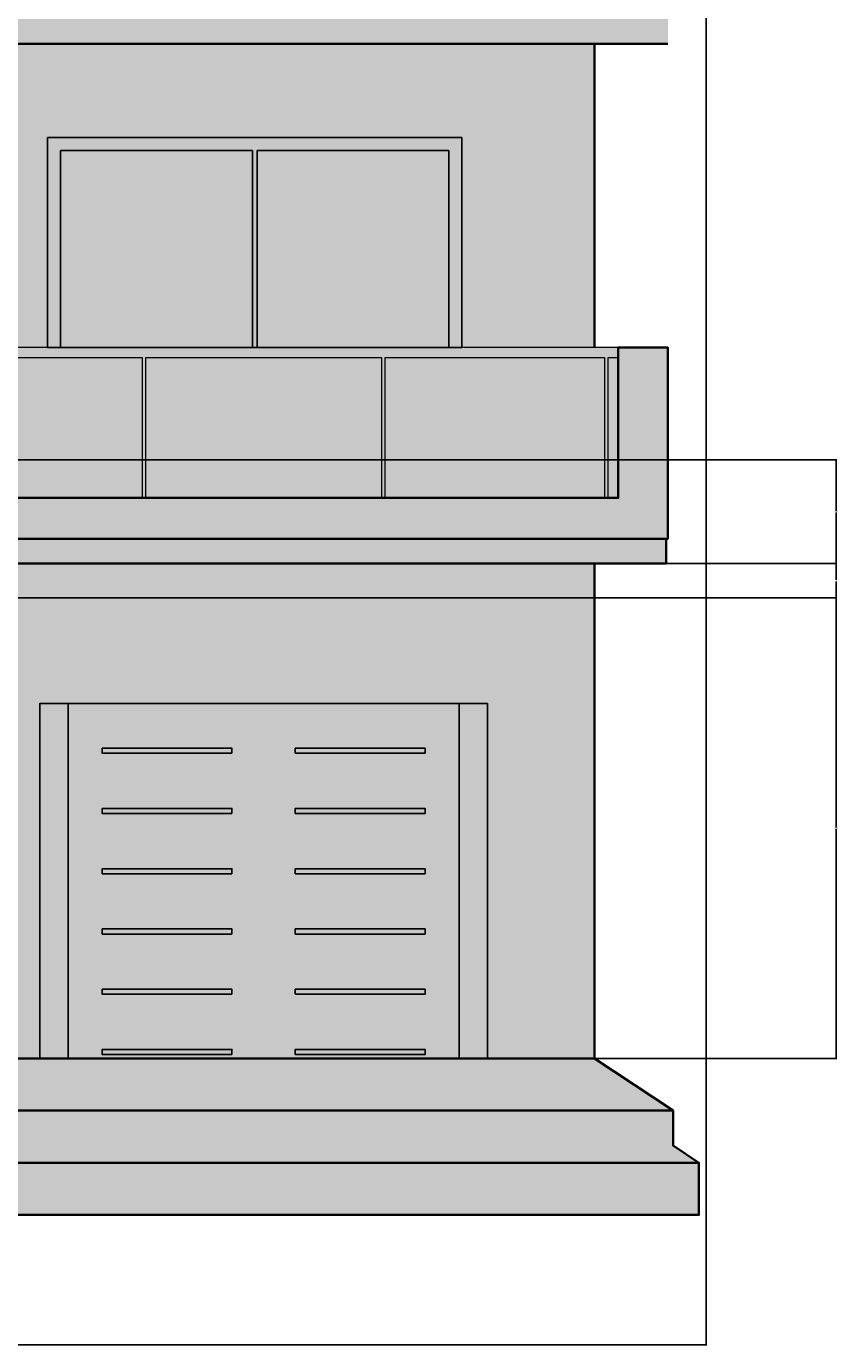
# Model space of a CAD drawing. Units: feet. Extents: x 2893 to 4112, y 897 to 1573.
# Tile 4 of 7: x 3253 to 3449, y 897 to 1217. Entities that reach past the tile are written whole.
import ezdxf

# ---------------------------------------------------------------- set-up
doc = ezdxf.new("R2010")
doc.units = ezdxf.units.FT
for name, color, linetype, lineweight in [('A-ANNO-DIMS', 2, 'Continuous', 18), ('A-DOOR', 3, 'Continuous', 25), ('A-ELEV', 7, 'Continuous', 35), ('A-ELEV-PATT', 8, 'Continuous', 13), ('A-ELEV-RAIL', 4, 'Continuous', 18), ('A-GLAZ', 4, 'Continuous', 25)]:
    doc.layers.add(name, color=color, linetype=linetype, lineweight=lineweight)
doc.styles.get("Standard").update_dxf_attribs({"font": 'arial.ttf'})
doc.dimstyles.get("Standard").update_dxf_attribs({"dimtxt": 0.18, "dimasz": 0.18, "dimexe": 0.18, "dimexo": 0.0625, "dimgap": 0.09, "dimtad": 0, "dimtih": 1, "dimtoh": 1, "dimdec": 1, "dimzin": 0, "dimdsep": 46, "dimlunit": 3, "dimtxsty": 'Standard', "dimcen": 0.09, "dimadec": 0, "dimazin": 0, "dimtfac": 1, "dimtdec": 1, "dimtofl": 0, "dimtmove": 0, "dimatfit": 3, "dimfxl": 1, "dimtolj": 1, "dimtzin": 0, "dimarcsym": 0})

# ---------------------------------------------------------------- blocks, each defined once
blk = doc.blocks.new('WIN-SLIDING')
blk.add_lwpolyline([(100.48, 0), (0, 0), (0, 50.91), (100.48, 50.91)], close=True)
blk.add_lwpolyline([(100.48, 0), (0, 0), (0, 50.91), (100.48, 50.91)], close=True)
blk.add_lwpolyline([(97.33, 0), (97.33, 47.76), (50.81, 47.76), (50.81, 0), (49.67, 0), (49.67, 47.76), (3.15, 47.76), (3.15, 0)])
blk.add_lwpolyline([(97.33, 0), (97.33, 47.76), (50.81, 47.76), (50.81, 0), (49.67, 0), (49.67, 47.76), (3.15, 47.76), (3.15, 0)])
blk = doc.blocks.new('GATE-GARAGE')
for points in [[(108.58, 0), (0, 0), (0, 86.02), (108.58, 86.02)], [(108.58, 0), (0, 0), (0, 86.02), (108.58, 86.02)], [(0, 86.02), (6.87, 86.02), (6.87, 0), (0, 0)], [(0, 86.02), (6.87, 86.02), (6.87, 0), (0, 0)], [(108.58, 86.02), (101.71, 86.02), (101.71, 0), (108.58, 0)], [(108.58, 86.02), (101.71, 86.02), (101.71, 0), (108.58, 0)], [(46.6, 73.98), (15.13, 73.98), (15.13, 75.22), (46.6, 75.22)], [(46.6, 73.98), (15.13, 73.98), (15.13, 75.22), (46.6, 75.22)], [(61.97, 73.98), (93.45, 73.98), (93.45, 75.22), (61.97, 75.22)], [(61.97, 73.98), (93.45, 73.98), (93.45, 75.22), (61.97, 75.22)], [(46.6, 59.37), (15.13, 59.37), (15.13, 60.61), (46.6, 60.61)], [(46.6, 59.37), (15.13, 59.37), (15.13, 60.61), (46.6, 60.61)], [(61.97, 59.37), (93.45, 59.37), (93.45, 60.61), (61.97, 60.61)], [(61.97, 59.37), (93.45, 59.37), (93.45, 60.61), (61.97, 60.61)], [(46.6, 44.76), (15.13, 44.76), (15.13, 46), (46.6, 46)], [(46.6, 44.76), (15.13, 44.76), (15.13, 46), (46.6, 46)], [(61.97, 44.76), (93.45, 44.76), (93.45, 46), (61.97, 46)], [(61.97, 44.76), (93.45, 44.76), (93.45, 46), (61.97, 46)], [(46.6, 30.15), (15.13, 30.15), (15.13, 31.39), (46.6, 31.39)], [(46.6, 30.15), (15.13, 30.15), (15.13, 31.39), (46.6, 31.39)], [(61.97, 30.15), (93.45, 30.15), (93.45, 31.39), (61.97, 31.39)], [(61.97, 30.15), (93.45, 30.15), (93.45, 31.39), (61.97, 31.39)], [(46.6, 15.54), (15.13, 15.54), (15.13, 16.78), (46.6, 16.78)], [(46.6, 15.54), (15.13, 15.54), (15.13, 16.78), (46.6, 16.78)], [(61.97, 15.54), (93.45, 15.54), (93.45, 16.78), (61.97, 16.78)], [(61.97, 15.54), (93.45, 15.54), (93.45, 16.78), (61.97, 16.78)], [(46.6, 0.93), (15.13, 0.93), (15.13, 2.17), (46.6, 2.17)], [(46.6, 0.93), (15.13, 0.93), (15.13, 2.17), (46.6, 2.17)], [(61.97, 0.93), (93.45, 0.93), (93.45, 2.17), (61.97, 2.17)], [(61.97, 0.93), (93.45, 0.93), (93.45, 2.17), (61.97, 2.17)]]:
    blk.add_lwpolyline(points, close=True)
blk = doc.blocks.new('BALCONY-RAIL')
blk.add_lwpolyline([(56.56, 34.07), (3.3, 34.07), (3.3, 0), (2.43, 0), (2.43, 34.07), (0, 34.07), (0, 36.45), (173.25, 36.45), (173.25, 34.07), (170.48, 34.07), (170.48, 0), (169.61, 0), (169.61, 34.07), (115.47, 34.07), (115.47, 0), (114.59, 0), (114.59, 34.07), (57.43, 34.07), (57.43, 0), (56.56, 0)], close=True)
blk.add_lwpolyline([(56.56, 34.07), (3.3, 34.07), (3.3, 0), (2.43, 0), (2.43, 34.07), (0, 34.07), (0, 36.45), (173.25, 36.45), (173.25, 34.07), (170.48, 34.07), (170.48, 0), (169.61, 0), (169.61, 34.07), (115.47, 34.07), (115.47, 0), (114.59, 0), (114.59, 34.07), (57.43, 34.07), (57.43, 0), (56.56, 0)], close=True)
blk = doc.blocks.new('*D48')
at = {"layer": 'A-ANNO-DIMS', "color": 0, "lineweight": -2, "transparency": 16777216}
for p, q in [((2924.72, 1491.83), (2924.72, 897.37)), ((3417.56, 1491.83), (3417.56, 897.37)), ((2924.9, 897.55), (3170.74, 897.55)), ((3417.38, 897.55), (3171.54, 897.55))]:
    blk.add_line(p, q, dxfattribs=at)
at = {"layer": 'A-ANNO-DIMS', "color": 0, "transparency": 16777216}
for points in [[(2924.9, 897.58), (2924.9, 897.52), (2924.72, 897.55)], [(3417.38, 897.58), (3417.38, 897.52), (3417.56, 897.55)]]:
    blk.add_solid(points, dxfattribs=at)
at = {"layer": 'Defpoints', "color": 0, "transparency": 16777216}
for p in [(2924.72, 1491.89), (3417.56, 1491.89), (3417.56, 897.55)]:
    blk.add_point(p, dxfattribs=at)
at = {"layer": 'A-ANNO-DIMS', "color": 0, "transparency": 16777216, "insert": (3171.14, 897.55), "char_height": 0.18, "attachment_point": 5}
blk.add_mtext('\\A1;492.8', dxfattribs=at)
blk = doc.blocks.new('*D49')
at = {"layer": 'A-ANNO-DIMS', "color": 0, "lineweight": -2, "transparency": 16777216}
for p, q in [((3215.03, 1078.68), (3449.24, 1078.68)), ((3449.06, 1078.5), (3449.06, 1023.03)), ((3449.06, 967.19), (3449.06, 1022.66)), ((3215.03, 967.01), (3449.24, 967.01))]:
    blk.add_line(p, q, dxfattribs=at)
at = {"layer": 'A-ANNO-DIMS', "color": 0, "transparency": 16777216}
for points in [[(3449.03, 1078.5), (3449.09, 1078.5), (3449.06, 1078.68)], [(3449.03, 967.19), (3449.09, 967.19), (3449.06, 967.01)]]:
    blk.add_solid(points, dxfattribs=at)
at = {"layer": 'Defpoints', "color": 0, "transparency": 16777216}
for p in [(3214.97, 1078.68), (3449.06, 1078.68), (3214.97, 967.01)]:
    blk.add_point(p, dxfattribs=at)
at = {"layer": 'A-ANNO-DIMS', "color": 0, "transparency": 16777216, "insert": (3449.06, 1022.85), "char_height": 0.18, "attachment_point": 5}
blk.add_mtext('\\A1;111.66', dxfattribs=at)
blk = doc.blocks.new('*D50')
at = {"layer": 'A-ANNO-DIMS', "color": 0, "lineweight": -2, "transparency": 16777216}
for p, q in [((3215.03, 1087.01), (3449.24, 1087.01)), ((3449.06, 1086.83), (3449.06, 1083.03)), ((3449.06, 1078.86), (3449.06, 1082.66)), ((3215.03, 1078.68), (3449.24, 1078.68))]:
    blk.add_line(p, q, dxfattribs=at)
at = {"layer": 'A-ANNO-DIMS', "color": 0, "transparency": 16777216}
for points in [[(3449.03, 1086.83), (3449.09, 1086.83), (3449.06, 1087.01)], [(3449.03, 1078.86), (3449.09, 1078.86), (3449.06, 1078.68)]]:
    blk.add_solid(points, dxfattribs=at)
at = {"layer": 'Defpoints', "color": 0, "transparency": 16777216}
for p in [(3214.97, 1087.01), (3449.06, 1087.01), (3214.97, 1078.68)]:
    blk.add_point(p, dxfattribs=at)
at = {"layer": 'A-ANNO-DIMS', "color": 0, "transparency": 16777216, "insert": (3449.06, 1082.85), "char_height": 0.18, "attachment_point": 5}
blk.add_mtext('\\A1;8.338', dxfattribs=at)
blk = doc.blocks.new('*D51')
at = {"layer": 'A-ANNO-DIMS', "color": 0, "lineweight": -2, "transparency": 16777216}
for p, q in [((3189.38, 1112.11), (3449.24, 1112.11)), ((3449.06, 1111.93), (3449.06, 1099.74)), ((3449.06, 1087.19), (3449.06, 1099.38)), ((3215.03, 1087.01), (3449.24, 1087.01))]:
    blk.add_line(p, q, dxfattribs=at)
at = {"layer": 'A-ANNO-DIMS', "color": 0, "transparency": 16777216}
for points in [[(3449.03, 1111.93), (3449.09, 1111.93), (3449.06, 1112.11)], [(3449.03, 1087.19), (3449.09, 1087.19), (3449.06, 1087.01)]]:
    blk.add_solid(points, dxfattribs=at)
at = {"layer": 'Defpoints', "color": 0, "transparency": 16777216}
for p in [(3189.32, 1112.11), (3449.06, 1112.11), (3214.97, 1087.01)]:
    blk.add_point(p, dxfattribs=at)
at = {"layer": 'A-ANNO-DIMS', "color": 0, "transparency": 16777216, "insert": (3449.06, 1099.56), "char_height": 0.18, "attachment_point": 5}
blk.add_mtext('\\A1;25.095', dxfattribs=at)

msp = doc.modelspace()

# ---------------------------------------------------------------- hatches: boundary and pattern name
at = {"layer": 'A-ELEV-PATT'}
h = msp.add_hatch(color=256, dxfattribs=at)
h.dxf.hatch_style = 1
h.paths.add_polyline_path([(3119.3255, 1527.889), (2924.7207, 1527.889), (2924.7207, 1491.889), (3119.3255, 1491.889)])
h.paths.add_polyline_path([(3417.5637, 1527.889), (3222.9589, 1527.889), (3222.9589, 1491.889), (3417.5637, 1491.889)])
h.paths.add_polyline_path([(3119.3255, 1102.9302), (2946.0771, 1102.9302), (2946.0771, 1139.3799), (2934.0287, 1139.3799), (2934.0287, 1093.0143), (3119.3255, 1093.0143)])
h.paths.add_polyline_path([(3119.3255, 1093.0143), (2934.4679, 1093.0143), (2934.4679, 1087.0143), (3119.3255, 1087.0143)])
h.paths.add_polyline_path([(3408.2557, 1139.3799), (3396.2073, 1139.3799), (3396.2073, 1136.9984), (3396.2073, 1102.9302), (3222.9589, 1102.9302), (3222.9589, 1093.0143), (3408.2557, 1093.0143)])
h.paths.add_polyline_path([(3407.8165, 1093.0143), (3222.9589, 1093.0143), (3222.9589, 1087.0143), (3407.8165, 1087.0143)])
h = msp.add_hatch(color=256, dxfattribs=at)
h.dxf.hatch_style = 1
h.paths.add_polyline_path([(3119.3255, 1491.889), (2924.7207, 1491.889), (2945.7801, 1471.0143), (3119.3255, 1471.0143)])
h.paths.add_polyline_path([(3119.3255, 1471.0143), (2945.7801, 1471.0143), (2951.8333, 1465.0143), (3119.3255, 1465.0143)])
h.paths.add_polyline_path([(3119.3255, 1465.0143), (2951.8333, 1465.0143), (2951.8333, 1381.4641), (2984.02, 1381.4641), (2984.02, 1432.3761), (3084.4999, 1432.3761), (3084.4999, 1381.4641), (3119.3255, 1381.4641)])
h.paths.add_polyline_path([(3417.5637, 1491.889), (3222.9589, 1491.889), (3222.9589, 1471.0143), (3396.5042, 1471.0143)])
h.paths.add_polyline_path([(3396.5042, 1471.0143), (3222.9589, 1471.0143), (3222.9589, 1465.0143), (3390.4511, 1465.0143)])
h.paths.add_polyline_path([(3390.4511, 1465.0143), (3222.9589, 1465.0143), (3222.9589, 1381.4641), (3257.7845, 1381.4641), (3257.7845, 1432.3761), (3358.2644, 1432.3761), (3358.2644, 1381.4641), (3390.4511, 1381.4641)])
h.paths.add_polyline_path([(3119.3255, 1339.0143), (2942.6825, 1339.0143), (2942.6825, 1232.1197), (2948.5078, 1232.1197), (2948.5078, 1266.188), (2946.0771, 1266.188), (2946.0771, 1268.5695), (2984.02, 1268.5695), (2984.02, 1319.4815), (3084.4999, 1319.4815), (3084.4999, 1268.5695), (3119.3255, 1268.5695)], flags=17)
h.paths.add_polyline_path([(3399.6019, 1339.0143), (3222.9589, 1339.0143), (3222.9589, 1268.5695), (3257.7845, 1268.5695), (3257.7845, 1319.4815), (3358.2644, 1319.4815), (3358.2644, 1268.5695), (3396.2073, 1268.5695), (3396.2073, 1266.188), (3393.7766, 1266.188), (3393.7766, 1232.1197), (3399.6019, 1232.1197)], flags=17)
h.paths.add_polyline_path([(2942.6825, 1339.0143), (3119.3255, 1339.0143), (3119.3255, 1345.0143), (2933.3946, 1345.0143), (2933.3946, 1232.1197), (2933.3946, 1220.0947), (3119.3255, 1220.0947), (3119.3255, 1232.1197), (2942.6825, 1232.1197)])
h.paths.add_polyline_path([(3408.8898, 1345.0143), (3222.9589, 1345.0143), (3222.9589, 1339.0143), (3399.6019, 1339.0143), (3399.6019, 1232.1197), (3393.7766, 1232.1197), (3392.9028, 1232.1197), (3222.9589, 1232.1197), (3222.9589, 1220.0947), (3408.8898, 1220.0947), (3408.8898, 1232.1197)])
h.paths.add_polyline_path([(2984.02, 1190.2919), (3084.4999, 1190.2919), (3084.4999, 1139.3799), (3119.3255, 1139.3799), (3119.3255, 1213.0143), (2951.8333, 1213.0143), (2951.8333, 1139.3799), (2984.02, 1139.3799)])
h.paths.add_polyline_path([(3119.3255, 1219.0143), (2934.0287, 1219.0143), (2951.8333, 1213.0143), (3119.3255, 1213.0143)])
h.paths.add_polyline_path([(3390.4511, 1213.0143), (3222.9589, 1213.0143), (3222.9589, 1139.3799), (3257.7845, 1139.3799), (3257.7845, 1190.2919), (3358.2644, 1190.2919), (3358.2644, 1139.3799), (3390.4511, 1139.3799)])
h.paths.add_polyline_path([(3408.2557, 1219.0143), (3222.9589, 1219.0143), (3222.9589, 1213.0143), (3408.2557, 1213.0143)])
h = msp.add_hatch(color=256, dxfattribs=at)
h.dxf.hatch_style = 1
h.paths.add_polyline_path([(3119.3255, 1139.3799), (2946.0771, 1139.3799), (2946.0771, 1136.9984), (2948.5078, 1136.9984), (2948.5078, 1102.9302), (2949.3816, 1102.9302), (2949.3816, 1136.9984), (3002.6337, 1136.9984), (3002.6337, 1102.9302), (3003.5075, 1102.9302), (3003.5075, 1136.9984), (3060.6708, 1136.9984), (3060.6708, 1102.9302), (3061.5445, 1102.9302), (3061.5445, 1136.9984), (3115.685, 1136.9984), (3115.685, 1102.9302), (3116.5588, 1102.9302), (3116.5588, 1136.9984), (3119.3255, 1136.9984)])
h.paths.add_polyline_path([(2987.1701, 1187.1419), (3033.6877, 1187.1419), (3033.6877, 1139.3799), (3034.8322, 1139.3799), (3034.8322, 1187.1419), (3081.3499, 1187.1419), (3081.3499, 1139.3799), (3084.4999, 1139.3799), (3084.4999, 1190.2919), (2984.02, 1190.2919), (2984.02, 1139.3799), (2987.1701, 1139.3799)])
h.paths.add_polyline_path([(2987.1701, 1316.3314), (3033.6877, 1316.3314), (3033.6877, 1268.5695), (3034.8322, 1268.5695), (3034.8322, 1316.3314), (3081.3499, 1316.3314), (3081.3499, 1268.5695), (3084.4999, 1268.5695), (3084.4999, 1319.4815), (2984.02, 1319.4815), (2984.02, 1268.5695), (2987.1701, 1268.5695)])
h.paths.add_polyline_path([(3003.5075, 1266.188), (3060.6708, 1266.188), (3060.6708, 1232.1197), (3061.5445, 1232.1197), (3061.5445, 1266.188), (3115.685, 1266.188), (3115.685, 1232.1197), (3116.5588, 1232.1197), (3116.5588, 1266.188), (3119.3255, 1266.188), (3119.3255, 1268.5695), (2946.0771, 1268.5695), (2946.0771, 1266.188), (2948.5078, 1266.188), (2948.5078, 1232.1197), (2949.3816, 1232.1197), (2949.3816, 1266.188), (3002.6337, 1266.188), (3002.6337, 1232.1197), (3003.5075, 1232.1197)])
h.paths.add_polyline_path([(2987.1701, 1429.226), (3033.6877, 1429.226), (3033.6877, 1381.4641), (3034.8322, 1381.4641), (3034.8322, 1429.226), (3081.3499, 1429.226), (3081.3499, 1381.4641), (3084.4999, 1381.4641), (3084.4999, 1432.3761), (2984.02, 1432.3761), (2984.02, 1381.4641), (2987.1701, 1381.4641)])
h.paths.add_polyline_path([(3119.3255, 1381.4641), (2946.0771, 1381.4641), (2946.0771, 1379.0826), (2948.5078, 1379.0826), (2948.5078, 1345.0143), (2949.3816, 1345.0143), (2949.3816, 1379.0826), (3002.6337, 1379.0826), (3002.6337, 1345.0143), (3003.5075, 1345.0143), (3003.5075, 1379.0826), (3060.6708, 1379.0826), (3060.6708, 1345.0143), (3061.5445, 1345.0143), (3061.5445, 1379.0826), (3115.685, 1379.0826), (3115.685, 1345.0143), (3116.5588, 1345.0143), (3116.5588, 1379.0826), (3119.3255, 1379.0826)])
h.paths.add_polyline_path([(3189.3169, 1482.3616), (3152.9675, 1482.3616), (3152.9675, 1457.0324), (3189.3169, 1457.0324)])
h.paths.add_polyline_path([(3155.237, 1480.0922), (3187.0474, 1480.0922), (3187.0474, 1459.3019), (3155.237, 1459.3019)], flags=16)
h.paths.add_polyline_path([(3189.3169, 1457.0324), (3152.9675, 1457.0324), (3152.9675, 1377.2236), (3189.3169, 1377.2236)])
h.paths.add_polyline_path([(3155.237, 1454.7629), (3187.0474, 1454.7629), (3187.0474, 1379.4931), (3155.237, 1379.4931)], flags=16)
h.paths.add_polyline_path([(3358.2644, 1432.3761), (3257.7845, 1432.3761), (3257.7845, 1381.4641), (3260.9345, 1381.4641), (3260.9345, 1429.226), (3307.4522, 1429.226), (3307.4522, 1381.4641), (3308.5967, 1381.4641), (3308.5967, 1429.226), (3355.1143, 1429.226), (3355.1143, 1381.4641), (3358.2644, 1381.4641)])
h.paths.add_polyline_path([(3396.2073, 1381.4641), (3222.9589, 1381.4641), (3222.9589, 1379.0826), (3225.7256, 1379.0826), (3225.7256, 1345.0143), (3226.5994, 1345.0143), (3226.5994, 1379.0826), (3280.7398, 1379.0826), (3280.7398, 1345.0143), (3281.6136, 1345.0143), (3281.6136, 1379.0826), (3338.7769, 1379.0826), (3338.7769, 1345.0143), (3339.6507, 1345.0143), (3339.6507, 1379.0826), (3392.9028, 1379.0826), (3392.9028, 1345.0143), (3393.7766, 1345.0143), (3393.7766, 1379.0826), (3396.2073, 1379.0826)])
h.paths.add_polyline_path([(3358.2644, 1319.4815), (3257.7845, 1319.4815), (3257.7845, 1268.5695), (3260.9345, 1268.5695), (3260.9345, 1316.3314), (3307.4522, 1316.3314), (3307.4522, 1268.5695), (3308.5967, 1268.5695), (3308.5967, 1316.3314), (3355.1143, 1316.3314), (3355.1143, 1268.5695), (3358.2644, 1268.5695)])
h.paths.add_polyline_path([(3396.2073, 1268.5695), (3222.9589, 1268.5695), (3222.9589, 1266.188), (3225.7256, 1266.188), (3225.7256, 1232.1197), (3226.5994, 1232.1197), (3226.5994, 1266.188), (3280.7398, 1266.188), (3280.7398, 1232.1197), (3281.6136, 1232.1197), (3281.6136, 1266.188), (3338.7769, 1266.188), (3338.7769, 1232.1197), (3339.6507, 1232.1197), (3339.6507, 1266.188), (3392.9028, 1266.188), (3392.9028, 1232.1197), (3393.7766, 1232.1197), (3393.7766, 1266.188), (3396.2073, 1266.188)])
h.paths.add_polyline_path([(3260.9345, 1187.1419), (3307.4522, 1187.1419), (3307.4522, 1139.3799), (3308.5967, 1139.3799), (3308.5967, 1187.1419), (3355.1143, 1187.1419), (3355.1143, 1139.3799), (3358.2644, 1139.3799), (3358.2644, 1190.2919), (3257.7845, 1190.2919), (3257.7845, 1139.3799), (3260.9345, 1139.3799)])
h.paths.add_polyline_path([(3396.2073, 1139.3799), (3222.9589, 1139.3799), (3222.9589, 1136.9984), (3225.7256, 1136.9984), (3225.7256, 1102.9302), (3226.5994, 1102.9302), (3226.5994, 1136.9984), (3280.7398, 1136.9984), (3280.7398, 1102.9302), (3281.6136, 1102.9302), (3281.6136, 1136.9984), (3338.7769, 1136.9984), (3338.7769, 1102.9302), (3339.6507, 1102.9302), (3339.6507, 1136.9984), (3392.9028, 1136.9984), (3392.9028, 1102.9302), (3393.7766, 1102.9302), (3393.7766, 1136.9984), (3396.2073, 1136.9984)])
h.paths.add_polyline_path([(3189.3169, 1354.8437), (3152.9675, 1354.8437), (3152.9675, 1329.5145), (3189.3169, 1329.5145)])
h.paths.add_polyline_path([(3155.237, 1331.784), (3155.237, 1352.5742), (3187.0474, 1352.5742), (3187.0474, 1331.784)], flags=16)
h.paths.add_polyline_path([(3189.3169, 1329.5145), (3152.9675, 1329.5145), (3152.9675, 1249.7057), (3189.3169, 1249.7057)])
h.paths.add_polyline_path([(3155.237, 1327.245), (3187.0474, 1327.245), (3187.0474, 1251.9752), (3155.237, 1251.9752)], flags=16)
h.paths.add_polyline_path([(3189.3169, 1191.9186), (3152.9675, 1191.9186), (3152.9675, 1112.1098), (3189.3169, 1112.1098)])
h.paths.add_polyline_path([(3155.237, 1189.6491), (3187.0474, 1189.6491), (3187.0474, 1114.3793), (3155.237, 1114.3793)], flags=16)
h.paths.add_polyline_path([(3189.3169, 1217.2478), (3152.9675, 1217.2478), (3152.9675, 1191.9186), (3189.3169, 1191.9186)])
h.paths.add_polyline_path([(3155.237, 1194.1881), (3155.237, 1214.9783), (3187.0474, 1214.9783), (3187.0474, 1194.1881)], flags=16)
h = msp.add_hatch(color=256, dxfattribs=at)
h.dxf.hatch_style = 1
h.paths.add_polyline_path([(3033.6877, 1429.226), (2987.1701, 1429.226), (2987.1701, 1381.4641), (3033.6877, 1381.4641)])
h.paths.add_polyline_path([(3081.3499, 1429.226), (3034.8322, 1429.226), (3034.8322, 1381.4641), (3081.3499, 1381.4641)])
h.paths.add_polyline_path([(3115.685, 1379.0826), (3061.5445, 1379.0826), (3061.5445, 1345.0143), (3115.685, 1345.0143)])
h.paths.add_polyline_path([(3119.3255, 1379.0826), (3116.5588, 1379.0826), (3116.5588, 1345.0143), (3119.3255, 1345.0143)])
h.paths.add_polyline_path([(3060.6708, 1379.0826), (3003.5075, 1379.0826), (3003.5075, 1345.0143), (3060.6708, 1345.0143)])
h.paths.add_polyline_path([(3002.6337, 1379.0826), (2949.3816, 1379.0826), (2949.3816, 1345.0143), (3002.6337, 1345.0143)])
h.paths.add_polyline_path([(2948.5078, 1379.0826), (2946.0771, 1379.0826), (2946.0771, 1345.0143), (2948.5078, 1345.0143)])
h.paths.add_polyline_path([(3355.1143, 1429.226), (3308.5967, 1429.226), (3308.5967, 1381.4641), (3355.1143, 1381.4641)])
h.paths.add_polyline_path([(3307.4522, 1429.226), (3260.9345, 1429.226), (3260.9345, 1381.4641), (3307.4522, 1381.4641)])
h.paths.add_polyline_path([(3225.7256, 1379.0826), (3222.9589, 1379.0826), (3222.9589, 1345.0143), (3225.7256, 1345.0143)])
h.paths.add_polyline_path([(3280.7398, 1379.0826), (3226.5994, 1379.0826), (3226.5994, 1345.0143), (3280.7398, 1345.0143)])
h.paths.add_polyline_path([(3338.7769, 1379.0826), (3281.6136, 1379.0826), (3281.6136, 1345.0143), (3338.7769, 1345.0143)])
h.paths.add_polyline_path([(3392.9028, 1379.0826), (3339.6507, 1379.0826), (3339.6507, 1345.0143), (3392.9028, 1345.0143)])
h.paths.add_polyline_path([(3187.0474, 1480.0922), (3155.237, 1480.0922), (3155.237, 1459.3019), (3187.0474, 1459.3019)])
h.paths.add_polyline_path([(3187.0474, 1454.7629), (3155.237, 1454.7629), (3155.237, 1379.4931), (3187.0474, 1379.4931)])
h.paths.add_polyline_path([(3187.0474, 1352.5742), (3155.237, 1352.5742), (3155.237, 1331.784), (3187.0474, 1331.784)])
h.paths.add_polyline_path([(3187.0474, 1327.245), (3155.237, 1327.245), (3155.237, 1251.9752), (3187.0474, 1251.9752)])
h.paths.add_polyline_path([(3033.6877, 1316.3314), (2987.1701, 1316.3314), (2987.1701, 1268.5695), (3033.6877, 1268.5695)])
h.paths.add_polyline_path([(3081.3499, 1316.3314), (3034.8322, 1316.3314), (3034.8322, 1268.5695), (3081.3499, 1268.5695)])
h.paths.add_polyline_path([(3002.6337, 1266.188), (2949.3816, 1266.188), (2949.3816, 1232.1197), (3002.6337, 1232.1197)])
h.paths.add_polyline_path([(3060.6708, 1266.188), (3003.5075, 1266.188), (3003.5075, 1232.1197), (3060.6708, 1232.1197)])
h.paths.add_polyline_path([(3115.685, 1266.188), (3061.5445, 1266.188), (3061.5445, 1232.1197), (3115.685, 1232.1197)])
h.paths.add_polyline_path([(3119.3255, 1266.188), (3116.5588, 1266.188), (3116.5588, 1232.1197), (3119.3255, 1232.1197)])
h.paths.add_polyline_path([(3307.4522, 1316.3314), (3260.9345, 1316.3314), (3260.9345, 1268.5695), (3307.4522, 1268.5695)])
h.paths.add_polyline_path([(3355.1143, 1316.3314), (3308.5967, 1316.3314), (3308.5967, 1268.5695), (3355.1143, 1268.5695)])
h.paths.add_polyline_path([(3392.9028, 1266.188), (3339.6507, 1266.188), (3339.6507, 1232.1197), (3392.9028, 1232.1197)])
h.paths.add_polyline_path([(3338.7769, 1266.188), (3281.6136, 1266.188), (3281.6136, 1232.1197), (3338.7769, 1232.1197)])
h.paths.add_polyline_path([(3280.7398, 1266.188), (3226.5994, 1266.188), (3226.5994, 1232.1197), (3280.7398, 1232.1197)])
h.paths.add_polyline_path([(3225.7256, 1266.188), (3222.9589, 1266.188), (3222.9589, 1232.1197), (3225.7256, 1232.1197)])
h.paths.add_polyline_path([(3033.6877, 1187.1419), (2987.1701, 1187.1419), (2987.1701, 1139.3799), (3033.6877, 1139.3799)])
h.paths.add_polyline_path([(3081.3499, 1187.1419), (3034.8322, 1187.1419), (3034.8322, 1139.3799), (3081.3499, 1139.3799)])
h.paths.add_polyline_path([(3002.6337, 1136.9984), (2949.3816, 1136.9984), (2949.3816, 1102.9302), (3002.6337, 1102.9302)])
h.paths.add_polyline_path([(3060.6708, 1136.9984), (3003.5075, 1136.9984), (3003.5075, 1102.9302), (3060.6708, 1102.9302)])
h.paths.add_polyline_path([(3115.685, 1136.9984), (3061.5445, 1136.9984), (3061.5445, 1102.9302), (3115.685, 1102.9302)])
h.paths.add_polyline_path([(3187.0474, 1214.9783), (3155.237, 1214.9783), (3155.237, 1194.1881), (3187.0474, 1194.1881)])
h.paths.add_polyline_path([(3187.0474, 1189.6491), (3155.237, 1189.6491), (3155.237, 1114.3793), (3187.0474, 1114.3793)])
h.paths.add_polyline_path([(3307.4522, 1187.1419), (3260.9345, 1187.1419), (3260.9345, 1139.3799), (3307.4522, 1139.3799)])
h.paths.add_polyline_path([(3355.1143, 1187.1419), (3308.5967, 1187.1419), (3308.5967, 1139.3799), (3355.1143, 1139.3799)])
h.paths.add_polyline_path([(3280.7398, 1136.9984), (3226.5994, 1136.9984), (3226.5994, 1102.9302), (3280.7398, 1102.9302)])
h.paths.add_polyline_path([(3338.7769, 1136.9984), (3281.6136, 1136.9984), (3281.6136, 1102.9302), (3338.7769, 1102.9302)])
h.paths.add_polyline_path([(3392.9028, 1136.9984), (3339.6507, 1136.9984), (3339.6507, 1102.9302), (3392.9028, 1102.9302)])
h.paths.add_polyline_path([(3225.7256, 1136.9984), (3222.9589, 1136.9984), (3222.9589, 1102.9302), (3225.7256, 1102.9302)])
h.paths.add_polyline_path([(3119.3255, 1136.9984), (3116.5588, 1136.9984), (3116.5588, 1102.9302), (3119.3255, 1102.9302)])
h.paths.add_polyline_path([(2948.5078, 1136.9984), (2946.0771, 1136.9984), (2946.0771, 1102.9302), (2948.5078, 1102.9302)])
h.paths.add_polyline_path([(3396.2073, 1136.9984), (3393.7766, 1136.9984), (3393.7766, 1102.9302), (3396.2073, 1102.9302)])
h = msp.add_hatch(color=256, dxfattribs=at)
h.dxf.hatch_style = 1
h.paths.add_polyline_path([(3390.4511, 1087.0143), (3222.9589, 1087.0143), (3222.9589, 967.0143), (3255.8959, 967.0143), (3255.8959, 1053.0375), (3262.7641, 1053.0375), (3364.4735, 1053.0375), (3364.4735, 967.0143), (3390.4511, 967.0143)])
h.paths.add_polyline_path([(3119.3255, 1087.0143), (2951.8333, 1087.0143), (2951.8333, 967.0143), (2977.8109, 967.0143), (2977.8109, 1053.0375), (2984.6791, 1053.0375), (3086.3885, 1053.0375), (3086.3885, 967.0143), (3119.3255, 967.0143)])
h = msp.add_hatch(color=256, dxfattribs=at)
h.dxf.hatch_style = 1
h.paths.add_polyline_path([(3079.5203, 1053.0375), (2984.6791, 1053.0375), (2984.6791, 967.0143), (3079.5203, 967.0143)])
h.paths.add_polyline_path([(3024.4136, 1040.9943), (2992.942, 1040.9943), (2992.942, 1042.2356), (3024.4136, 1042.2356)], flags=16)
h.paths.add_polyline_path([(3039.7858, 1042.2356), (3071.2574, 1042.2356), (3071.2574, 1040.9943), (3039.7858, 1040.9943)], flags=16)
h.paths.add_polyline_path([(3024.4136, 1027.6246), (3024.4136, 1026.3833), (2992.942, 1026.3833), (2992.942, 1027.6246)], flags=16)
h.paths.add_polyline_path([(3039.7858, 1027.6246), (3071.2574, 1027.6246), (3071.2574, 1026.3833), (3039.7858, 1026.3833)], flags=16)
h.paths.add_polyline_path([(3024.4136, 1013.0137), (3024.4136, 1011.7724), (2992.942, 1011.7724), (2992.942, 1013.0137)], flags=16)
h.paths.add_polyline_path([(3039.7858, 1013.0137), (3071.2574, 1013.0137), (3071.2574, 1011.7724), (3039.7858, 1011.7724)], flags=16)
h.paths.add_polyline_path([(3024.4136, 998.4028), (3024.4136, 997.1615), (2992.942, 997.1615), (2992.942, 998.4028)], flags=16)
h.paths.add_polyline_path([(3039.7858, 998.4028), (3071.2574, 998.4028), (3071.2574, 997.1615), (3039.7858, 997.1615)], flags=16)
h.paths.add_polyline_path([(3024.4136, 983.7919), (3024.4136, 982.5506), (2992.942, 982.5506), (2992.942, 983.7919)], flags=16)
h.paths.add_polyline_path([(3039.7858, 983.7919), (3071.2574, 983.7919), (3071.2574, 982.5506), (3039.7858, 982.5506)], flags=16)
h.paths.add_polyline_path([(3024.4136, 969.181), (3024.4136, 967.9397), (2992.942, 967.9397), (2992.942, 969.181)], flags=16)
h.paths.add_polyline_path([(3039.7858, 969.181), (3071.2574, 969.181), (3071.2574, 967.9397), (3039.7858, 967.9397)], flags=16)
h.paths.add_polyline_path([(3086.3885, 1053.0375), (3079.5203, 1053.0375), (3079.5203, 967.0143), (3086.3885, 967.0143)])
h.paths.add_polyline_path([(3364.4735, 1053.0375), (3357.6053, 1053.0375), (3357.6053, 967.0143), (3364.4735, 967.0143)])
h.paths.add_polyline_path([(3357.6053, 1053.0375), (3262.7641, 1053.0375), (3262.7641, 967.0143), (3357.6053, 967.0143)])
h.paths.add_polyline_path([(3271.027, 1026.3833), (3271.027, 1027.6246), (3302.4986, 1027.6246), (3302.4986, 1026.3833)], flags=16)
h.paths.add_polyline_path([(3271.027, 1013.0137), (3302.4986, 1013.0137), (3302.4986, 1011.7724), (3271.027, 1011.7724)], flags=16)
h.paths.add_polyline_path([(3271.027, 1040.9943), (3271.027, 1042.2356), (3302.4986, 1042.2356), (3302.4986, 1040.9943)], flags=16)
h.paths.add_polyline_path([(3271.027, 998.4028), (3302.4986, 998.4028), (3302.4986, 997.1615), (3271.027, 997.1615)], flags=16)
h.paths.add_polyline_path([(3271.027, 983.7919), (3302.4986, 983.7919), (3302.4986, 982.5506), (3271.027, 982.5506)], flags=16)
h.paths.add_polyline_path([(3317.8708, 1026.3833), (3317.8708, 1027.6246), (3349.3424, 1027.6246), (3349.3424, 1026.3833)], flags=16)
h.paths.add_polyline_path([(3317.8708, 1013.0137), (3349.3424, 1013.0137), (3349.3424, 1011.7724), (3317.8708, 1011.7724)], flags=16)
h.paths.add_polyline_path([(3271.027, 969.181), (3302.4986, 969.181), (3302.4986, 967.9397), (3271.027, 967.9397)], flags=16)
h.paths.add_polyline_path([(3317.8708, 1040.9943), (3317.8708, 1042.2356), (3349.3424, 1042.2356), (3349.3424, 1040.9943)], flags=16)
h.paths.add_polyline_path([(3317.8708, 998.4028), (3349.3424, 998.4028), (3349.3424, 997.1615), (3317.8708, 997.1615)], flags=16)
h.paths.add_polyline_path([(3317.8708, 983.7919), (3349.3424, 983.7919), (3349.3424, 982.5506), (3317.8708, 982.5506)], flags=16)
h.paths.add_polyline_path([(3317.8708, 969.181), (3349.3424, 969.181), (3349.3424, 967.9397), (3317.8708, 967.9397)], flags=16)
h.paths.add_polyline_path([(3262.7641, 1053.0375), (3255.8959, 1053.0375), (3255.8959, 967.0143), (3262.7641, 967.0143)])
h.paths.add_polyline_path([(2984.6791, 1053.0375), (2977.8109, 1053.0375), (2977.8109, 967.0143), (2984.6791, 967.0143)])
h = msp.add_hatch(color=256, dxfattribs=at)
h.dxf.hatch_style = 1
h.paths.add_polyline_path([(3024.4136, 1042.2356), (2992.942, 1042.2356), (2992.942, 1040.9943), (3024.4136, 1040.9943)])
h.paths.add_polyline_path([(3071.2574, 1042.2356), (3039.7858, 1042.2356), (3039.7858, 1040.9943), (3071.2574, 1040.9943)])
h.paths.add_polyline_path([(3024.4136, 1027.6246), (2992.942, 1027.6246), (2992.942, 1026.3833), (3024.4136, 1026.3833)])
h.paths.add_polyline_path([(3071.2574, 1027.6246), (3039.7858, 1027.6246), (3039.7858, 1026.3833), (3071.2574, 1026.3833)])
h.paths.add_polyline_path([(3024.4136, 1013.0137), (2992.942, 1013.0137), (2992.942, 1011.7724), (3024.4136, 1011.7724)])
h.paths.add_polyline_path([(3071.2574, 1013.0137), (3039.7858, 1013.0137), (3039.7858, 1011.7724), (3071.2574, 1011.7724)])
h.paths.add_polyline_path([(3024.4136, 998.4028), (2992.942, 998.4028), (2992.942, 997.1615), (3024.4136, 997.1615)])
h.paths.add_polyline_path([(3071.2574, 998.4028), (3039.7858, 998.4028), (3039.7858, 997.1615), (3071.2574, 997.1615)])
h.paths.add_polyline_path([(3024.4136, 983.7919), (2992.942, 983.7919), (2992.942, 982.5506), (3024.4136, 982.5506)])
h.paths.add_polyline_path([(3071.2574, 983.7919), (3039.7858, 983.7919), (3039.7858, 982.5506), (3071.2574, 982.5506)])
h.paths.add_polyline_path([(3071.2574, 969.181), (3039.7858, 969.181), (3039.7858, 967.9397), (3071.2574, 967.9397)])
h.paths.add_polyline_path([(3024.4136, 969.181), (2992.942, 969.181), (2992.942, 967.9397), (3024.4136, 967.9397)])
h.paths.add_polyline_path([(3302.4986, 1042.2356), (3271.027, 1042.2356), (3271.027, 1040.9943), (3302.4986, 1040.9943)])
h.paths.add_polyline_path([(3349.3424, 1042.2356), (3317.8708, 1042.2356), (3317.8708, 1040.9943), (3349.3424, 1040.9943)])
h.paths.add_polyline_path([(3302.4986, 1027.6246), (3271.027, 1027.6246), (3271.027, 1026.3833), (3302.4986, 1026.3833)])
h.paths.add_polyline_path([(3349.3424, 1027.6246), (3317.8708, 1027.6246), (3317.8708, 1026.3833), (3349.3424, 1026.3833)])
h.paths.add_polyline_path([(3302.4986, 1013.0137), (3271.027, 1013.0137), (3271.027, 1011.7724), (3302.4986, 1011.7724)])
h.paths.add_polyline_path([(3349.3424, 1013.0137), (3317.8708, 1013.0137), (3317.8708, 1011.7724), (3349.3424, 1011.7724)])
h.paths.add_polyline_path([(3302.4986, 998.4028), (3271.027, 998.4028), (3271.027, 997.1615), (3302.4986, 997.1615)])
h.paths.add_polyline_path([(3349.3424, 998.4028), (3317.8708, 998.4028), (3317.8708, 997.1615), (3349.3424, 997.1615)])
h.paths.add_polyline_path([(3302.4986, 983.7919), (3271.027, 983.7919), (3271.027, 982.5506), (3302.4986, 982.5506)])
h.paths.add_polyline_path([(3349.3424, 983.7919), (3317.8708, 983.7919), (3317.8708, 982.5506), (3349.3424, 982.5506)])
h.paths.add_polyline_path([(3302.4986, 969.181), (3271.027, 969.181), (3271.027, 967.9397), (3302.4986, 967.9397)])
h.paths.add_polyline_path([(3349.3424, 969.181), (3317.8708, 969.181), (3317.8708, 967.9397), (3349.3424, 967.9397)])
h = msp.add_hatch(color=256, dxfattribs=at)
h.dxf.hatch_style = 1
h.paths.add_polyline_path([(3390.4511, 967.0143), (3222.9589, 967.0143), (2951.8333, 967.0143), (2932.7702, 954.3595), (3409.5142, 954.3595)])
h.paths.add_polyline_path([(3409.5142, 954.3595), (2932.7702, 954.3595), (2932.7702, 945.8624), (2926.5072, 941.7047), (3415.7772, 941.7047), (3409.5142, 945.8624)])
h.paths.add_polyline_path([(3415.7772, 941.7047), (2926.5072, 941.7047), (2926.5072, 929.0499), (3415.7772, 929.0499)])

# ---------------------------------------------------------------- linework, layer by layer
at = {"layer": 'A-ELEV'}
for p, q in [((3222.9589, 1213.0143), (3408.2557, 1213.0143)), ((3222.9589, 1213.0143), (3408.2557, 1213.0143)), ((3390.4511, 1213.0143), (3390.4511, 1139.3799)), ((3390.4511, 1213.0143), (3390.4511, 1139.3799)), ((3222.9589, 1093.0143), (3408.2557, 1093.0143)), ((3407.8165, 1087.0143), (3222.9589, 1087.0143)), ((2951.8333, 967.0143), (3390.4511, 967.0143)), ((2951.8333, 967.0143), (3390.4511, 967.0143)), ((3409.5142, 954.3595), (3390.4511, 967.0143)), ((3409.5142, 954.3595), (3390.4511, 967.0143)), ((3415.7772, 941.7047), (3409.5142, 945.8624)), ((3415.7772, 941.7047), (3415.7772, 929.0499))]:
    msp.add_line(p, q, dxfattribs=at)
for points in [[(3222.9589, 1093.0143), (3408.2557, 1093.0143), (3408.2557, 1139.3799), (3396.2073, 1139.3799), (3396.2073, 1102.9302), (3222.9589, 1102.9302), (3222.9589, 1087.0143), (3407.8165, 1087.0143), (3407.8165, 1093.0143)], [(3396.2073, 1102.9302), (3396.2073, 1139.3799), (3408.2557, 1139.3799), (3408.2557, 1093.0143)], [(3222.9589, 1087.0143), (3222.9589, 1102.9302), (3396.2073, 1102.9302)], [(3407.8165, 1087.0143), (3407.8165, 1093.0143)], [(2932.7702, 945.8624), (2932.7702, 954.3595), (3409.5142, 954.3595), (3409.5142, 945.8624)], [(2926.5072, 941.7047), (3415.7772, 941.7047)], [(2926.5072, 941.7047), (3415.7772, 941.7047)], [(3409.5142, 941.7047), (2932.7702, 941.7047)], [(3409.5142, 941.7047), (2932.7702, 941.7047)], [(3415.7772, 929.0499), (2926.5072, 929.0499)]]:
    msp.add_lwpolyline(points, dxfattribs=at)
for points in [[(3390.4511, 967.0143), (3222.9589, 967.0143), (3222.9589, 1087.0143), (3390.4511, 1087.0143)], [(3390.4511, 967.0143), (3222.9589, 967.0143), (3222.9589, 1087.0143), (3390.4511, 1087.0143)], [(2926.5072, 941.7047), (2932.7702, 945.8624), (2932.7702, 954.3595), (3409.5142, 954.3595), (3409.5142, 945.8624), (3415.7772, 941.7047), (3415.7772, 929.0499), (2926.5072, 929.0499)]]:
    msp.add_lwpolyline(points, close=True, dxfattribs=at)

# ---------------------------------------------------------------- block references
at = {"layer": 'A-DOOR', "extrusion": (0, 0, -1), "zscale": -1}
msp.add_blockref('GATE-GARAGE', (-3364.4734, 967.014), dxfattribs=at)
at = {"layer": 'A-ELEV-RAIL', "extrusion": (0, 0, -1), "zscale": -1}
msp.add_blockref('BALCONY-RAIL', (-3396.2074, 1102.93), dxfattribs=at)
at = {"layer": 'A-GLAZ', "extrusion": (0, 0, -1), "zscale": -1}
msp.add_blockref('WIN-SLIDING', (-3358.2644, 1139.38), dxfattribs=at)

# ---------------------------------------------------------------- dimensions: what is measured, and where the dimension line sits
at = {"layer": 'A-ANNO-DIMS'}
dim = msp.add_linear_dim(base=(3417.5637, 897.5499), p1=(2924.7207, 1491.889), p2=(3417.5637, 1491.889), dimstyle='Standard', override={"dimdec": 1, "dimlfac": 1, "dimrnd": 0, "dimzin": 0, "dimdsep": 46, "dimlunit": 2}, dxfattribs=at)
dim.commit()
dim.dimension.update_dxf_attribs({"geometry": '*D48', "text_midpoint": (3171.1422, 897.5499)})
for base, p1, p2, override, picture, middle in [((3449.06374, 1112.1098), (3214.96934, 1087.01433), (3189.3169, 1112.1098), {"dimdec": 3, "dimlfac": 1, "dimrnd": 0, "dimzin": 0, "dimdsep": 46, "dimlunit": 2}, '*D51', (3449.06374, 1099.56206)), ((3449.0637, 1087.0143), (3214.9693, 1078.6766), (3214.9693, 1087.0143), {"dimdec": 3, "dimlfac": 1, "dimrnd": 0, "dimzin": 0, "dimdsep": 46, "dimlunit": 2}, '*D50', (3449.0637, 1082.8455)), ((3449.0637, 1078.6766), (3214.9693, 967.0143), (3214.9693, 1078.6766), {"dimdec": 2, "dimlfac": 1, "dimrnd": 0, "dimzin": 0, "dimdsep": 46, "dimlunit": 2}, '*D49', (3449.0637, 1022.8455))]:
    dim = msp.add_linear_dim(base=base, p1=p1, p2=p2, angle=90, dimstyle='Standard', override=override, dxfattribs=at)
    dim.commit()
    dim.dimension.update_dxf_attribs({"geometry": picture, "text_midpoint": middle})

doc.saveas('drawing.dxf')
